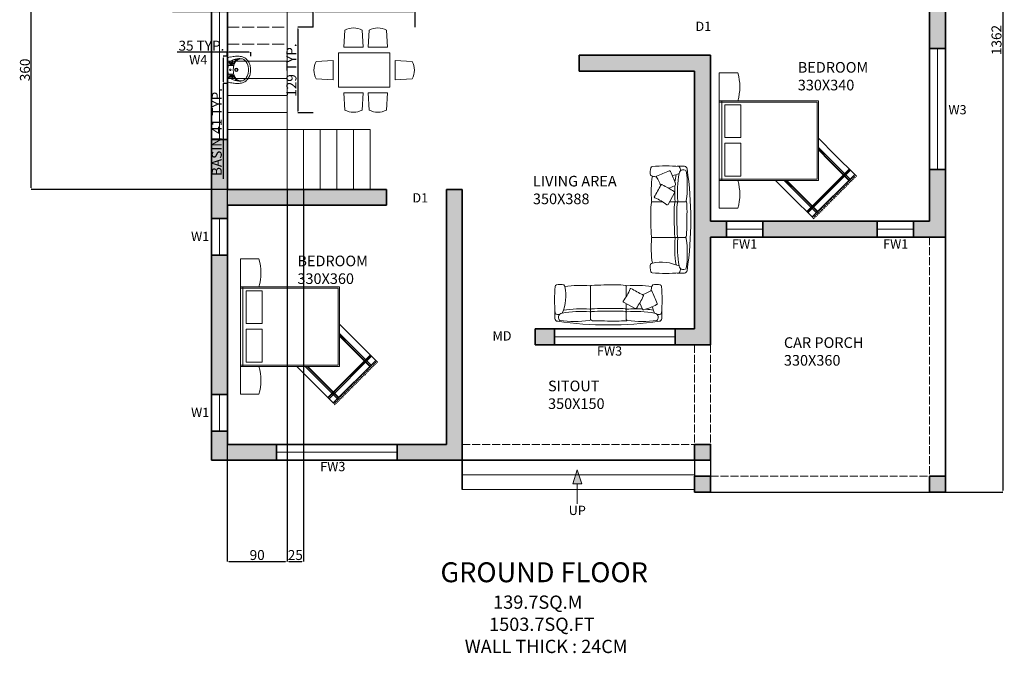
# Model space of a CAD drawing. Units: centimetres. Extents: x 2449 to 7478, y 778 to 2486.
# Tile 5 of 9: x 4189 to 5672, y 778 to 1732. Entities that reach past the tile are written whole.
import ezdxf

# ---------------------------------------------------------------- set-up
doc = ezdxf.new("R2010")
doc.units = ezdxf.units.CM
doc.linetypes.add('ACAD_ISO02W100', pattern=[15, 12, -3])
for name, color, linetype, lineweight in [('0.15', 34, 'Continuous', 15), ('A-ANNO-DIMS', 2, 'Continuous', 18), ('A-ANNO-SYMB', 8, 'Continuous', 18), ('A-ANNO-TEXT', 7, 'Continuous', 18), ('A-ANNO-TITL', 7, 'Continuous', 25), ('A-AREA-IDEN', 7, 'Continuous', 18), ('A-COLS', 7, 'Continuous', 35), ('A-COLS-PATT', 7, 'Continuous', 13), ('A-FLOR', 7, 'Continuous', 25), ('A-FLOR-FIXT', 8, 'Continuous', 18), ('A-FLOR-OVHD', 8, 'ACAD_ISO02W100', 18), ('A-FLOR-STRS', 7, 'Continuous', 18), ('A-FLOR-STRS-OVHD', 7, 'ACAD_ISO02W100', 13), ('A-WALL', 7, 'Continuous', 35), ('A-WALL-PATT', 7, 'Continuous', 13), ('B-FURNITURE', 22, 'Continuous', 18), ('Win', 1, 'Continuous', 18)]:
    doc.layers.add(name, color=color, linetype=linetype, lineweight=lineweight)
doc.styles.get("Standard").update_dxf_attribs({"font": 'arial.ttf'})
doc.dimstyles.new('ISO-25', dxfattribs={"dimtxt": 15, "dimasz": 2.5, "dimexe": 0, "dimexo": 0, "dimgap": 0, "dimtad": 1, "dimtxsty": 'Standard', "dimcen": 2.5, "dimadec": 0, "dimazin": 0, "dimtfac": 1, "dimtmove": 0, "dimatfit": 3, "dimfxl": 1, "dimarcsym": 0})

# ---------------------------------------------------------------- blocks, each defined once
blk = doc.blocks.new('ролар')
at = {"layer": 'B-FURNITURE'}
for p, q in [((182149, -12928), (182149, -13090)), ((182946, -12908), (182946, -13070)), ((183742, -12908), (183742, -13070)), ((184538, -12927), (184538, -13090)), ((182946, -13070), (182946, -13655)), ((183742, -13070), (183742, -13261)), ((183742, -13412), (183742, -13655))]:
    blk.add_line(p, q, dxfattribs=at)
blk.add_lwpolyline([(184124, -13426, 0.039108), (183972, -13160, 0.352413), (183942, -13151), (183685, -13293, 0.370087), (183675, -13320, -0.085318), (183831, -13592, 0.338149), (183848, -13604, -0.006963), (184118, -13456, 0.478074)], format="xyb", close=True, dxfattribs=at)
blk.add_lwpolyline([(184112, -13464, -0.054969), (184295, -13552, 0.338149), (184316, -13550, -0.006963), (184437, -13268, 0.478074), (184423, -13240, 0.039108), (184140, -13125, 0.352413), (184110, -13136), (184052, -13272)], format="xyb", dxfattribs=at)
for centre, radius, start, end in [((182209, -12928), 60, 90, 180), ((183344, -20690), 7904, 81.7476, 98.2524), ((182322, -12954), 95.7, 154.4132, 226.8965), ((182264, -12914), 28.1, 104.7154, 176.7534), ((182585, -15161), 2298, 81.7903, 98.2097), ((182918, -12915), 28.9, 15.2961, 99.1888), ((182999, -12942), 63.3, 99.7658, 147.0241), ((181568, 80195), 93085, 270.87421, 271.20678), ((183296, -20822), 7955, 86.6979, 88.3256), ((183770, -12915), 28.9, 80.8112, 164.7039), ((184102, -15161), 2298, 81.7903, 98.2097), ((184423, -12914), 28.1, 3.2466, 75.2846), ((184365, -12954), 95.7, 313.1035, 25.5868), ((184478, -12928), 60, 358.6006, 89.9879), ((186046, -13346), 3905, 175.5762, 184.4238), ((182224, -13128), 110, 72.3508, 130.321), ((182340, -12922), 131, 230.7956, 255.727), ((181452, -13440), 941, 347.608, 24.5904), ((182727, -10699), 2387, 259.8888, 274.8671), ((182725, -10712), 2434, 260.7796, 274.8194), ((182927, -13057), 20.3, 275.8765, 1.8), ((182927, -13117), 20.3, 275.8765, 1.8), ((182962, -13065), 17.3, 149.88, 272.0041), ((182962, -13125), 17.3, 149.88, 272.0041), ((183401, -6361), 6736, 266.2761, 271.089), ((183401, -6421), 6736, 266.2761, 271.089), ((183573, -12278), 819, 266.8813, 280.6931), ((183573, -12338), 819, 266.8813, 280.6931), ((183725, -13065), 17.3, 267.9959, 30.12), ((183725, -13125), 17.3, 267.9959, 30.12), ((183760, -13057), 20.3, 178.2, 264.1235), ((183760, -13117), 20.3, 178.2, 264.1235), ((183961, -10699), 2387, 265.1329, 280.1112), ((184001, -9721), 3425, 265.9379, 271.7664), ((184034, -11509), 1637, 275.2593, 281.2487), ((185235, -13440), 941, 155.4096, 164.8885), ((184348, -12922), 131, 284.273, 309.2044), ((184464, -13128), 110, 49.679, 107.6492), ((180641, -13346), 3905, 355.5762, 4.4238), ((182195, -13642), 42.7, 187.075, 250.1971), ((181903, -13435), 512, 330.8359, 336.0732), ((182722, -11168), 2503, 261.8987, 274.7524), ((182927, -13643), 20.3, 275.8765, 1.8), ((182962, -13651), 17.3, 149.88, 272.0041), ((183725, -13651), 17.3, 267.9959, 30.12), ((183760, -13643), 20.3, 178.2, 264.1235), ((183966, -11168), 2503, 265.2476, 278.1013), ((185235, -13440), 941, 186.9661, 192.392), ((184785, -13435), 512, 203.9268, 209.1641), ((184493, -13642), 42.7, 289.8029, 352.925), ((182270, -13358), 336, 254.5718, 283.8571), ((183401, -6946), 6736, 266.2761, 271.089), ((183573, -12863), 819, 266.8813, 280.6931), ((184418, -13358), 336, 256.1429, 285.4282)]:
    blk.add_arc(centre, radius, start, end, dxfattribs=at)
blk = doc.blocks.new('table-11')
at = {"color": 0, "linetype": 'ByBlock'}
for p, q in [((-1.122, 0.533), (-1.144, 0.134)), ((-0.716, 0.533), (-0.694, 0.134)), ((-0.554, 0.533), (-0.576, 0.134)), ((-0.148, 0.533), (-0.126, 0.134)), ((0, 0), (-1.2, 0)), ((-1.2, -0.8), (-1.2, 0)), ((-1.144, 0.134), (-0.694, 0.134)), ((-0.576, 0.134), (-0.126, 0.134)), ((0, -0.8), (0, 0)), ((-1.723, -0.197), (-1.324, -0.175)), ((-1.324, -0.625), (-1.324, -0.175)), ((0.523, -0.197), (0.124, -0.175)), ((0.124, -0.625), (0.124, -0.175)), ((-1.723, -0.603), (-1.324, -0.625)), ((0.523, -0.603), (0.124, -0.625)), ((0, -0.8), (-1.2, -0.8)), ((-1.144, -0.934), (-0.694, -0.934)), ((-1.122, -1.333), (-1.144, -0.934)), ((-0.716, -1.333), (-0.694, -0.934)), ((-0.576, -0.934), (-0.126, -0.934)), ((-0.554, -1.333), (-0.576, -0.934)), ((-0.148, -1.333), (-0.126, -0.934))]:
    blk.add_line(p, q, dxfattribs=at)
for centre, start, end in [((-0.919, 0.159), 61.4891, 118.5109), ((-0.351, 0.159), 61.4891, 118.5109), ((-1.349, -0.4), 151.4891, 208.5109), ((0.149, -0.4), 331.4891, 28.5109), ((-0.919, -0.959), 241.4891, 298.5109), ((-0.351, -0.959), 241.4891, 298.5109)]:
    blk.add_arc(centre, 0.425, start, end, dxfattribs=at)
blk = doc.blocks.new('A$C376C2187')
at = {"layer": 'B-FURNITURE'}
for p, q in [((-1.53, 1.82), (-1.53, 2.24)), ((-1.53, 2.24), (-0.9, 2.24)), ((-0.9, 0), (-0.9, 2.24)), ((-0.9, 2.24), (0.9, 2.24)), ((-0.9, 2.24), (-0.9, 1.82)), ((-0.87, 0.03), (-0.87, 2.24)), ((0.87, 2.24), (0.87, 0.03)), ((0.9, 2.24), (0.9, 0)), ((0.9, 1.82), (0.9, 2.24)), ((0.9, 2.24), (1.53, 2.24)), ((1.53, 2.24), (1.53, 1.82)), ((-0.9, 2.182), (0.9, 2.182)), ((-0.807, 2.112), (-0.057, 2.112)), ((-0.807, 1.749), (-0.807, 2.112)), ((-0.057, 2.112), (-0.057, 1.749)), ((0.069, 2.112), (0.807, 2.112)), ((0.069, 2.112), (0.069, 1.749)), ((0.807, 2.112), (0.807, 1.749)), ((-0.807, 1.749), (-0.057, 1.749)), ((0.069, 1.749), (0.807, 1.749)), ((0.9, 0), (-0.9, 0)), ((0.87, 0.03), (-0.87, 0.03))]:
    blk.add_line(p, q, dxfattribs=at)
for centre in [(-1.215, 2.926), (1.215, 2.926)]:
    blk.add_arc(centre, 1.15, 254.0965, 285.9035, dxfattribs=at)
blk = doc.blocks.new('lavamanos 2')
at = {"layer": '0.15'}
for p, q in [((0, 0.234), (0, -0.234)), ((-0.13, 0.11), (-0.131, 0.11)), ((-0.014, 0.087), (-0.13, 0.086)), ((-0.113, 0.112), (-0.107, 0.158)), ((-0.104, 0.111), (-0.098, 0.157)), ((-0.086, 0.109), (-0.081, 0.147)), ((-0.077, 0.107), (-0.072, 0.145)), ((-0.059, 0.105), (-0.055, 0.135)), ((-0.05, 0.104), (-0.046, 0.134)), ((-0.13, -0.11), (-0.131, -0.11)), ((-0.014, -0.087), (-0.13, -0.086)), ((-0.113, -0.112), (-0.107, -0.158)), ((-0.104, -0.111), (-0.098, -0.157)), ((-0.086, -0.109), (-0.081, -0.147)), ((-0.077, -0.107), (-0.072, -0.145)), ((-0.059, -0.105), (-0.055, -0.135)), ((-0.05, -0.104), (-0.046, -0.134))]:
    blk.add_line(p, q, dxfattribs=at)
for centre, radius in [((-0.178, 0), 0.035), ((-0.178, 0), 0.0235), ((-0.06, 0), 0.015)]:
    blk.add_circle(centre, radius, dxfattribs=at)
for centre, radius, start, end in [((-0.166, 0.001), 0.302, 136.5719, 154.3277), ((-0.242, 0.066), 0.202, 108.1945, 135.3686), ((-0.242, 0.065), 0.164, 121.9929, 150.5889), ((-0.266, 0.104), 0.119, 92.4774, 122.1411), ((-0.203, -0.086), 0.359, 91.203, 106.4255), ((-0.277, 0.068), 0.153, 57.2491, 95.54), ((-0.244, -0.013), 0.237, 77.2482, 96.4632), ((-0.221, -0.685), 0.959, 86.5514, 89.4131), ((-0.277, 0.068), 0.168, 56.8766, 64.9971), ((-0.222, 0.003), 0.218, 71.9849, 82.0124), ((-0.366, -0.002), 0.278, 40.3525, 49.2255), ((-0.212, -0.548), 0.82, 83.1224, 86.5796), ((-0.31, -0.315), 0.547, 69.5191, 73.4912), ((-0.299, -0.285), 0.516, 65.23, 69.5378), ((5.828, 30.215), 30.532, 258.7782, 258.876), ((-0.126, -0.066), 0.329, 69.0601, 78.8218), ((-0.02, 0.212), 0.0314, 54.7949, 69.0601), ((-0.005, 0.234), 0.005, 0, 54.7949), ((-0.209, 0.006), 0.256, 171.3102, 181.2627), ((-0.209, -0.006), 0.256, 178.7373, 188.6898), ((-0.056, -0.018), 0.411, 158.7011, 171.3102), ((0.466, -0.083), 0.895, 169.8632, 174.658), ((0.466, 0.083), 0.895, 185.342, 190.1368), ((-0.2, 0.026), 0.22, 147.1156, 167.4425), ((-0.366, -0.002), 0.263, 40.3525, 49.0046), ((-0.237, 0.11), 0.0921, 27.3186, 39.1156), ((-0.349, 0.036), 0.226, 22.3361, 30.8927), ((-0.237, 0.11), 0.107, 27.5743, 39.1156), ((-0.349, 0.036), 0.241, 22.1921, 30.7838), ((-1.266, -0.239), 1.182, 16.3631, 17.7767), ((-0.132, 0.117), 0.007, 197.4099, 270.4949), ((0.185, 0.165), 0.325, 192.5389, 196.7072), ((-0.13, 0.117), 0.007, 270.4949, 17.3953), ((-1.266, -0.239), 1.197, 17.3953, 17.8049), ((0.389, 0.121), 0.517, 185.5053, 189.8131), ((-0.718, -0.007), 0.599, 0.6765, 3.8216), ((-0.718, 0.007), 0.599, 356.1784, 359.3235), ((-0.108, 0.111), 0.0045, 172.614, 352.614), ((-0.102, 0.158), 0.0045, 352.614, 172.614), ((-0.081, 0.108), 0.0045, 172.614, 352.614), ((-0.278, -0.241), 0.466, 60.2413, 65.2382), ((-0.076, 0.146), 0.0045, 352.614, 172.614), ((-0.054, 0.104), 0.0045, 172.614, 352.614), ((-0.05, 0.135), 0.0045, 352.614, 172.614), ((-0.065, 0.118), 0.049, 1.5827, 68.6208), ((-2.148, 0.001), 2.135, 359.9754, 3.1901), ((-2.148, -0.001), 2.135, 356.8099, 0.0246), ((-0.056, 0.018), 0.411, 188.6898, 201.2989), ((-0.166, -0.001), 0.302, 205.6723, 223.4281), ((-0.2, -0.026), 0.22, 192.5575, 212.8844), ((-0.242, -0.065), 0.164, 209.4111, 238.0071), ((-0.277, -0.068), 0.153, 264.46, 302.7509), ((-0.366, 0.002), 0.263, 310.9954, 319.6475), ((-0.366, 0.002), 0.278, 310.7745, 319.6475), ((-0.237, -0.11), 0.0921, 320.8844, 332.6814), ((-0.349, -0.036), 0.226, 329.1073, 337.6639), ((-0.237, -0.11), 0.107, 320.8844, 332.4257), ((-0.349, -0.036), 0.241, 329.2162, 337.8079), ((-1.266, 0.239), 1.182, 342.2233, 343.6369), ((-0.132, -0.117), 0.007, 89.5051, 162.5901), ((0.185, -0.165), 0.325, 163.2928, 167.4611), ((-0.13, -0.117), 0.007, 342.6047, 89.5051), ((0.389, -0.121), 0.517, 170.1869, 174.4947), ((-1.266, 0.239), 1.197, 342.1951, 342.6047), ((-0.299, 0.286), 0.516, 290.4622, 294.77), ((-0.108, -0.111), 0.0045, 7.386, 187.386), ((-0.102, -0.158), 0.0045, 187.386, 7.386), ((-0.081, -0.108), 0.0045, 7.386, 187.386), ((-0.278, 0.241), 0.466, 294.7618, 299.7587), ((-0.076, -0.146), 0.0045, 187.386, 7.386), ((-0.054, -0.104), 0.0045, 7.386, 187.386), ((-0.05, -0.135), 0.0045, 187.386, 7.386), ((-0.065, -0.118), 0.049, 291.3792, 358.4173), ((-0.242, -0.066), 0.202, 224.6314, 251.8055), ((-0.266, -0.104), 0.119, 237.8589, 267.5226), ((-0.203, 0.086), 0.359, 253.5745, 268.797), ((-0.244, 0.013), 0.237, 263.5368, 282.7518), ((-0.221, 0.685), 0.959, 270.5869, 273.4486), ((-0.277, -0.068), 0.168, 295.0029, 303.1234), ((-0.222, -0.003), 0.218, 277.9876, 288.0151), ((-0.212, 0.548), 0.82, 273.4204, 276.8776), ((-0.31, 0.315), 0.547, 286.5088, 290.4809), ((5.828, -30.215), 30.532, 101.124, 101.2218), ((-0.126, 0.066), 0.329, 281.1782, 290.9399), ((-0.02, -0.212), 0.0314, 290.9399, 305.2051), ((-0.005, -0.234), 0.005, 305.2051, 0)]:
    blk.add_arc(centre, radius, start, end, dxfattribs=at)
blk = doc.blocks.new('RUG-FRINGED-B')
for p, q in [((90.4, 95.2), (64.4, 121.3)), ((64.4, 107.4), (83.5, 88.3)), ((64.4, 104.7), (82.1, 86.9)), ((64.4, 103.6), (81.6, 86.3)), ((90.4, 95.2), (119.1, 66.6)), ((110.7, 74.9), (46.8, 11)), ((111.3, 74.4), (47.4, 10.4)), ((110.2, 57.7), (81.6, 86.3)), ((110.8, 58.3), (82.1, 86.9)), ((112.1, 59.7), (83.5, 88.3)), ((112.7, 73), (48.7, 9)), ((119.1, 66.6), (55.1, 2.7)), ((112.3, 59.9), (115, 57.3)), ((114, 61.6), (116.6, 58.9)), ((115.7, 63.2), (118.3, 60.6)), ((117.4, 64.9), (120, 62.3)), ((119.1, 66.6), (121.7, 64)), ((0, 57.8), (26.5, 31.3)), ((32.9, 37.7), (12.8, 57.8)), ((34.2, 39), (15.5, 57.8)), ((34.8, 39.6), (16.7, 57.8)), ((97.2, 44.8), (99.8, 42.1)), ((98.9, 46.4), (101.5, 43.8)), ((100.6, 48.1), (103.2, 45.5)), ((102.3, 49.8), (104.9, 47.2)), ((103.9, 51.5), (106.6, 48.9)), ((105.6, 53.2), (108.2, 50.5)), ((107.3, 54.8), (109.9, 52.2)), ((109, 56.5), (111.6, 53.9)), ((110.7, 58.2), (113.3, 55.6)), ((55.1, 2.7), (26.5, 31.3)), ((32.9, 37.7), (61.5, 9)), ((34.2, 39), (62.9, 10.4)), ((34.8, 39.6), (63.4, 11)), ((83.8, 31.3), (86.4, 28.7)), ((85.5, 33), (88.1, 30.4)), ((87.1, 34.7), (89.8, 32.1)), ((88.8, 36.4), (91.4, 33.7)), ((90.5, 38), (93.1, 35.4)), ((92.2, 39.7), (94.8, 37.1)), ((93.9, 41.4), (96.5, 38.8)), ((95.5, 43.1), (98.2, 40.5)), ((68.7, 16.2), (71.3, 13.6)), ((70.3, 17.9), (73, 15.3)), ((72, 19.6), (74.6, 16.9)), ((73.7, 21.2), (76.3, 18.6)), ((75.4, 22.9), (78, 20.3)), ((77.1, 24.6), (79.7, 22)), ((78.7, 26.3), (81.4, 23.7)), ((80.4, 28), (83, 25.3)), ((82.1, 29.6), (84.7, 27)), ((55.2, 2.8), (57.8, 0.1)), ((56.9, 4.4), (59.5, 1.8)), ((58.6, 6.1), (61.2, 3.5)), ((60.3, 7.8), (62.9, 5.2)), ((61.9, 9.5), (64.6, 6.9)), ((63.6, 11.2), (66.2, 8.5)), ((65.3, 12.8), (67.9, 10.2)), ((67, 14.5), (69.6, 11.9))]:
    blk.add_line(p, q)
for centre in [(118.4, 60.6), (120.1, 62.2), (121.8, 63.9), (103.3, 45.4), (105, 47.1), (106.6, 48.8), (108.3, 50.5), (110, 52.2), (111.7, 53.8), (113.4, 55.5), (115, 57.2), (116.7, 58.9), (88.1, 30.3), (89.8, 32), (91.5, 33.7), (93.2, 35.4), (94.9, 37), (96.5, 38.7), (98.2, 40.4), (99.9, 42.1), (101.6, 43.8), (73, 15.2), (74.7, 16.9), (76.4, 18.6), (78.1, 20.2), (79.7, 21.9), (81.4, 23.6), (83.1, 25.3), (84.8, 27), (86.5, 28.6), (57.9, 0.1), (59.6, 1.8), (61.3, 3.4), (62.9, 5.1), (64.6, 6.8), (66.3, 8.5), (68, 10.2), (69.7, 11.8), (71.3, 13.5)]:
    blk.add_circle(centre, 0.0789)
blk = doc.blocks.new('ARROW-ENTRY-UP')
at = {"transparency": 33554687}
h = blk.add_hatch(color=256, dxfattribs=at)
h.dxf.hatch_style = 1
h.paths.add_polyline_path([(-6.8, 30.3), (6.8, 30.3), (0, 51.2)])
blk.add_line((0, 30.3), (0, 0))
blk.add_lwpolyline([(0, 51.2), (-6.8, 30.3), (6.8, 30.3)], close=True)
blk = doc.blocks.new('*D88')
at = {"layer": 'A-ANNO-DIMS', "color": 0, "lineweight": -2, "transparency": 16777216}
for p, q in [((4630.8, 1743.6), (4418.6, 1743.6)), ((4630.8, 1720.5), (4630.8, 1743.6)), ((4781.9, 1743.6), (4633.3, 1743.6)), ((4784.4, 1720.5), (4784.4, 1743.6))]:
    blk.add_line(p, q, dxfattribs=at)
at = {"layer": 'A-ANNO-DIMS', "color": 0, "transparency": 16777216}
for points in [[(4633.3, 1744), (4633.3, 1743.2), (4630.8, 1743.6)], [(4781.9, 1744), (4781.9, 1743.2), (4784.4, 1743.6)]]:
    blk.add_solid(points, dxfattribs=at)
at = {"layer": 'Defpoints', "color": 0, "transparency": 16777216}
for p in [(4630.8, 1743.6), (4630.8, 1720.5), (4784.4, 1720.5)]:
    blk.add_point(p, dxfattribs=at)
at = {"layer": 'A-ANNO-DIMS', "color": 0, "transparency": 16777216, "insert": (4523.4, 1751.3), "char_height": 15, "attachment_point": 5}
blk.add_mtext('DINING SET 154 TYP.', dxfattribs=at)
blk = doc.blocks.new('*D89')
at = {"layer": 'A-ANNO-DIMS', "color": 0, "lineweight": -2, "transparency": 16777216}
for p, q in [((4630.8, 1720.5), (4607.7, 1720.5)), ((4607.7, 1718), (4607.7, 1593.9)), ((4630.8, 1591.4), (4607.7, 1591.4))]:
    blk.add_line(p, q, dxfattribs=at)
at = {"layer": 'A-ANNO-DIMS', "color": 0, "transparency": 16777216}
for points in [[(4607.3, 1718), (4608.1, 1718), (4607.7, 1720.5)], [(4607.3, 1593.9), (4608.1, 1593.9), (4607.7, 1591.4)]]:
    blk.add_solid(points, dxfattribs=at)
at = {"layer": 'Defpoints', "color": 0, "transparency": 16777216}
for p in [(4630.8, 1720.5), (4607.7, 1591.4), (4630.8, 1591.4)]:
    blk.add_point(p, dxfattribs=at)
at = {"layer": 'A-ANNO-DIMS', "color": 0, "transparency": 16777216, "insert": (4600, 1656), "char_height": 15, "attachment_point": 5, "rotation": 90}
blk.add_mtext('129 TYP.', dxfattribs=at)
blk = doc.blocks.new('*D94')
at = {"layer": 'A-ANNO-DIMS', "color": 0, "lineweight": -2, "transparency": 16777216}
for p, q in [((4501.4, 1676.9), (4495.3, 1676.9)), ((4495.3, 1674.4), (4495.3, 1638.2)), ((4501.4, 1635.7), (4495.3, 1635.7)), ((4495.3, 1635.7), (4495.3, 1492.2))]:
    blk.add_line(p, q, dxfattribs=at)
at = {"layer": 'A-ANNO-DIMS', "color": 0, "transparency": 16777216}
for points in [[(4494.9, 1674.4), (4495.7, 1674.4), (4495.3, 1676.9)], [(4494.9, 1638.2), (4495.7, 1638.2), (4495.3, 1635.7)]]:
    blk.add_solid(points, dxfattribs=at)
at = {"layer": 'Defpoints', "color": 0, "transparency": 16777216}
for p in [(4501.4, 1676.9), (4495.3, 1635.7), (4501.4, 1635.7)]:
    blk.add_point(p, dxfattribs=at)
at = {"layer": 'A-ANNO-DIMS', "color": 0, "transparency": 16777216, "insert": (4487.5, 1562.7), "char_height": 15, "attachment_point": 5, "rotation": 89.9999}
blk.add_mtext('BASIN 41 TYP.', dxfattribs=at)
blk = doc.blocks.new('*D95')
at = {"layer": 'A-ANNO-DIMS', "color": 0, "lineweight": -2, "transparency": 16777216}
for p, q in [((4501.4, 1683.1), (4425.9, 1683.1)), ((4501.4, 1676.9), (4501.4, 1683.1)), ((4534.1, 1683.1), (4503.9, 1683.1)), ((4536.6, 1676.9), (4536.6, 1683.1))]:
    blk.add_line(p, q, dxfattribs=at)
at = {"layer": 'A-ANNO-DIMS', "color": 0, "transparency": 16777216}
for points in [[(4503.9, 1683.5), (4503.9, 1682.7), (4501.4, 1683.1)], [(4534.1, 1683.5), (4534.1, 1682.7), (4536.6, 1683.1)]]:
    blk.add_solid(points, dxfattribs=at)
at = {"layer": 'Defpoints', "color": 0, "transparency": 16777216}
for p in [(4501.4, 1683.1), (4501.4, 1676.9), (4536.6, 1676.9)]:
    blk.add_point(p, dxfattribs=at)
at = {"layer": 'A-ANNO-DIMS', "color": 0, "transparency": 16777216, "insert": (4462.4, 1690.8), "char_height": 15, "attachment_point": 5, "rotation": 359.9999}
blk.add_mtext('35 TYP.', dxfattribs=at)
blk = doc.blocks.new('*D101')
at = {"layer": 'A-ANNO-DIMS', "color": 0, "lineweight": -2, "transparency": 16777216}
for p, q in [((5583.4, 2382.3), (5669.9, 2382.3)), ((5669.9, 2379.8), (5669.9, 1022.8)), ((5583.4, 1020.3), (5669.9, 1020.3))]:
    blk.add_line(p, q, dxfattribs=at)
at = {"layer": 'A-ANNO-DIMS', "color": 0, "transparency": 16777216}
for points in [[(5669.5, 2379.8), (5670.4, 2379.8), (5669.9, 2382.3)], [(5669.5, 1022.8), (5670.4, 1022.8), (5669.9, 1020.3)]]:
    blk.add_solid(points, dxfattribs=at)
at = {"layer": 'Defpoints', "color": 0, "transparency": 16777216}
for p in [(5583.4, 2382.3), (5583.4, 1020.3), (5669.9, 1020.3)]:
    blk.add_point(p, dxfattribs=at)
at = {"layer": 'A-ANNO-DIMS', "color": 0, "transparency": 16777216, "insert": (5662.3, 1701.3), "char_height": 15, "attachment_point": 5, "rotation": 90}
blk.add_mtext('1362', dxfattribs=at)
blk = doc.blocks.new('*D102')
at = {"layer": 'A-ANNO-DIMS', "color": 0, "lineweight": -2, "transparency": 16777216}
for p, q in [((4501.4, 1476.3), (4501.4, 916)), ((4591.4, 1476.3), (4591.4, 916)), ((4503.9, 916), (4588.9, 916))]:
    blk.add_line(p, q, dxfattribs=at)
at = {"layer": 'A-ANNO-DIMS', "color": 0, "transparency": 16777216}
for points in [[(4503.9, 916.4), (4503.9, 915.6), (4501.4, 916)], [(4588.9, 916.4), (4588.9, 915.6), (4591.4, 916)]]:
    blk.add_solid(points, dxfattribs=at)
at = {"layer": 'Defpoints', "color": 0, "transparency": 16777216}
for p in [(4501.4, 1476.3), (4591.4, 1476.3), (4591.4, 916)]:
    blk.add_point(p, dxfattribs=at)
at = {"layer": 'A-ANNO-DIMS', "color": 0, "transparency": 16777216, "insert": (4546.4, 923.7), "char_height": 15, "attachment_point": 5}
blk.add_mtext('90', dxfattribs=at)
blk = doc.blocks.new('*D103')
at = {"layer": 'A-ANNO-DIMS', "color": 0, "lineweight": -2, "transparency": 16777216}
for p, q in [((4591.4, 1476.3), (4591.4, 916)), ((4616.4, 1476.3), (4616.4, 916)), ((4593.9, 916), (4613.9, 916))]:
    blk.add_line(p, q, dxfattribs=at)
at = {"layer": 'A-ANNO-DIMS', "color": 0, "transparency": 16777216}
for points in [[(4593.9, 916.4), (4593.9, 915.6), (4591.4, 916)], [(4613.9, 916.4), (4613.9, 915.6), (4616.4, 916)]]:
    blk.add_solid(points, dxfattribs=at)
at = {"layer": 'Defpoints', "color": 0, "transparency": 16777216}
for p in [(4591.4, 1476.3), (4616.4, 1476.3), (4616.4, 916)]:
    blk.add_point(p, dxfattribs=at)
at = {"layer": 'A-ANNO-DIMS', "color": 0, "transparency": 16777216, "insert": (4603.9, 923.7), "char_height": 15, "attachment_point": 5}
blk.add_mtext('25', dxfattribs=at)
blk = doc.blocks.new('*D104')
at = {"layer": 'A-ANNO-DIMS', "color": 0, "lineweight": -2, "transparency": 16777216}
for p, q in [((4501.4, 1836.3), (4206.1, 1836.3)), ((4206.1, 1478.8), (4206.1, 1833.8)), ((4501.4, 1476.3), (4206.1, 1476.3))]:
    blk.add_line(p, q, dxfattribs=at)
at = {"layer": 'A-ANNO-DIMS', "color": 0, "transparency": 16777216}
for points in [[(4205.7, 1833.8), (4206.5, 1833.8), (4206.1, 1836.3)], [(4205.7, 1478.8), (4206.5, 1478.8), (4206.1, 1476.3)]]:
    blk.add_solid(points, dxfattribs=at)
at = {"layer": 'Defpoints', "color": 0, "transparency": 16777216}
for p in [(4206.1, 1836.3), (4501.4, 1836.3), (4501.4, 1476.3)]:
    blk.add_point(p, dxfattribs=at)
at = {"layer": 'A-ANNO-DIMS', "color": 0, "transparency": 16777216, "insert": (4198.4, 1656.3), "char_height": 15, "attachment_point": 5, "rotation": 90}
blk.add_mtext('360', dxfattribs=at)

msp = doc.modelspace()

# ---------------------------------------------------------------- hatches: boundary and pattern name
at = {"layer": 'A-COLS-PATT'}
h = msp.add_hatch(color=256, dxfattribs=at)
h.dxf.hatch_style = 1
h.paths.add_polyline_path([(5229.448, 1092.34), (5205.448, 1092.34), (5205.448, 1068.34), (5229.448, 1068.34)])
h = msp.add_hatch(color=256, dxfattribs=at)
h.dxf.hatch_style = 1
h.paths.add_polyline_path([(5205.448, 1020.34), (5229.448, 1020.34), (5229.448, 1044.34), (5205.448, 1044.34)])
h = msp.add_hatch(color=256, dxfattribs=at)
h.dxf.hatch_style = 1
h.paths.add_polyline_path([(5559.448, 1020.34), (5583.448, 1020.34), (5583.448, 1044.34), (5559.448, 1044.34)])
at = {"layer": 'A-WALL-PATT'}
h = msp.add_hatch(color=256, dxfattribs=at)
h.dxf.hatch_style = 1
h.paths.add_polyline_path([(4831.448, 1092.34), (4757.448, 1092.34), (4757.448, 1068.34), (4855.448, 1068.34), (4855.448, 1476.34), (4831.448, 1476.34)])
h.paths.add_polyline_path([(4477.448, 1167.34), (4501.448, 1167.34), (4501.448, 1377.34), (4477.448, 1377.34)])
h.paths.add_polyline_path([(4575.448, 1068.34), (4575.448, 1092.34), (4501.448, 1092.34), (4501.448, 1112.34), (4477.448, 1112.34), (4477.448, 1068.34)])
h.paths.add_polyline_path([(4501.448, 1551.34), (4477.448, 1551.34), (4477.448, 1432.34), (4501.448, 1432.34), (4501.448, 1452.34), (4741.448, 1452.34), (4741.448, 1476.34), (4501.448, 1476.34)])
h.paths.add_polyline_path([(5205.448, 1654.34), (5205.448, 1266.34), (5176.448, 1266.34), (5176.448, 1242.34), (5229.448, 1242.34), (5229.448, 1404.34), (5253.448, 1404.34), (5253.448, 1428.34), (5229.448, 1428.34), (5229.448, 1678.34), (5031.448, 1678.34), (5031.448, 1654.34)])
h.paths.add_polyline_path([(4994.448, 1266.34), (4965.448, 1266.34), (4965.448, 1242.34), (4994.448, 1242.34)])
h.paths.add_polyline_path([(5583.448, 1506.339), (5559.448, 1506.339), (5559.448, 1428.34), (5535.448, 1428.34), (5535.448, 1404.34), (5583.448, 1404.34)])
h.paths.add_polyline_path([(5480.448, 1404.34), (5480.448, 1428.34), (5308.448, 1428.34), (5308.448, 1404.34)])
h.paths.add_polyline_path([(5559.448, 1688.339), (5583.448, 1688.339), (5583.448, 1826.34), (5559.448, 1826.34), (5559.448, 1792.34), (5418.448, 1792.34), (5418.448, 1768.34), (5559.448, 1768.34)])
h.paths.add_polyline_path([(5559.448, 1956.34), (5319.448, 1956.34), (5319.448, 1792.34), (5205.448, 1792.34), (5205.448, 1768.34), (5343.448, 1768.34), (5343.448, 1932.34), (5559.448, 1932.34), (5559.448, 1898.34), (5583.448, 1898.34), (5583.448, 2065.339), (5559.448, 2065.339)])
h.paths.add_polyline_path([(5559.448, 2358.34), (5559.448, 2247.339), (5583.448, 2247.339), (5583.448, 2382.34), (5535.448, 2382.34), (5535.448, 2358.34)])
h.paths.add_polyline_path([(5308.448, 2382.34), (5308.448, 2358.34), (5480.448, 2358.34), (5480.448, 2382.34)])
h.paths.add_polyline_path([(5229.448, 2358.34), (5253.448, 2358.34), (5253.448, 2382.34), (5205.448, 2382.34), (5205.448, 2214.34), (5166.448, 2214.34), (5166.448, 2190.34), (5205.448, 2190.34), (5205.448, 2065.34), (5229.448, 2065.34)])
h.paths.add_polyline_path([(5002.448, 2214.34), (5002.448, 2190.34), (5031.448, 2190.34), (5031.448, 1966.34), (5205.448, 1966.34), (5205.448, 1932.34), (5229.448, 1932.34), (5229.448, 1990.34), (5055.448, 1990.34), (5055.448, 2190.34), (5094.448, 2190.34), (5094.448, 2214.34)])
h.paths.add_polyline_path([(4901.448, 2190.34), (4930.448, 2190.34), (4930.448, 2214.34), (4803.448, 2214.34), (4803.448, 2190.34), (4877.448, 2190.34), (4877.448, 1836.34), (4901.448, 1836.34), (4901.448, 1966.34), (4956.448, 1966.34), (4956.448, 1990.34), (4901.448, 1990.34)])
h.paths.add_polyline_path([(4509.448, 2214.34), (4509.448, 2190.34), (4523.448, 2190.34), (4523.448, 1935.34), (4547.448, 1935.34), (4547.448, 2190.34), (4621.448, 2190.34), (4621.448, 2214.34)])
h.paths.add_polyline_path([(4349.448, 2152.839), (4373.448, 2152.839), (4373.448, 2190.34), (4387.448, 2190.34), (4387.448, 2214.34), (4349.448, 2214.34)])
h.paths.add_polyline_path([(4349.448, 1935.34), (4373.448, 1935.34), (4373.448, 1970.839), (4349.448, 1970.839)])
h.paths.add_polyline_path([(4477.448, 1836.34), (4477.448, 1791.34), (4501.448, 1791.34), (4501.448, 1836.34), (4787.448, 1836.34), (4787.448, 1860.34), (4349.448, 1860.34), (4349.448, 1836.34)])

# ---------------------------------------------------------------- linework, layer by layer
at = {"layer": 'A-COLS'}
for points in [[(5205.448, 1068.34), (5229.448, 1068.34), (5229.448, 1092.34), (5205.448, 1092.34)], [(5205.448, 1020.34), (5229.448, 1020.34), (5229.448, 1044.34), (5205.448, 1044.34)], [(5559.448, 1020.34), (5583.448, 1020.34), (5583.448, 1044.34), (5559.448, 1044.34)]]:
    msp.add_lwpolyline(points, close=True, dxfattribs=at)
at = {"layer": 'A-FLOR'}
for p, q in [((5205.448, 1092.34), (5205.448, 1020.34)), ((5229.448, 1092.34), (5229.448, 1044.34)), ((5205.448, 1044.34), (5229.448, 1044.34)), ((5205.448, 1020.34), (5583.448, 1020.34))]:
    msp.add_line(p, q, dxfattribs=at)
at = {"layer": 'A-FLOR-OVHD'}
for p, q in [((5559.448, 1404.34), (5559.448, 1044.34)), ((5205.448, 1242.34), (5205.448, 1092.34)), ((5229.448, 1242.34), (5229.448, 1092.34)), ((4855.448, 1092.34), (5229.448, 1092.34)), ((5229.448, 1044.34), (5559.448, 1044.34))]:
    msp.add_line(p, q, dxfattribs=at)
at = {"layer": 'A-FLOR-STRS'}
for p, q in [((4591.448, 1836.34), (4591.448, 1476.34)), ((4501.448, 1669.21), (4591.448, 1669.21)), ((4501.448, 1643.47), (4591.448, 1643.47)), ((4501.448, 1617.76), (4591.448, 1617.76)), ((4501.448, 1592.05), (4591.448, 1592.05)), ((4501.448, 1566.34), (4716.448, 1566.34)), ((4616.448, 1566.34), (4616.448, 1476.34)), ((4641.448, 1566.34), (4641.448, 1476.34)), ((4666.448, 1566.34), (4666.448, 1476.34)), ((4691.448, 1566.34), (4691.448, 1476.34)), ((4716.448, 1566.34), (4716.448, 1476.34)), ((4855.448, 1046.34), (5205.448, 1046.34)), ((4855.448, 1024.34), (5205.448, 1024.34))]:
    msp.add_line(p, q, dxfattribs=at)
at = {"layer": 'A-FLOR-STRS-OVHD', "ltscale": 1.5}
for p, q in [((4501.448, 1720.63), (4591.448, 1720.63)), ((4501.448, 1694.92), (4591.448, 1694.92))]:
    msp.add_line(p, q, dxfattribs=at)
at = {"layer": 'A-WALL'}
for p, q in [((5583.448, 2382.34), (5583.448, 1020.34)), ((4477.448, 1836.34), (4477.448, 1068.34)), ((4501.448, 1836.34), (4501.448, 1476.34)), ((5559.448, 1768.34), (5559.448, 1428.34)), ((5031.448, 1678.34), (5031.448, 1654.34)), ((5031.448, 1678.34), (5229.448, 1678.34)), ((5229.448, 1678.34), (5229.448, 1428.34)), ((5559.448, 1688.339), (5583.448, 1688.339)), ((5031.448, 1654.34), (5205.448, 1654.34)), ((5205.448, 1654.34), (5205.448, 1266.34)), ((4501.448, 1551.34), (4477.448, 1551.34)), ((5559.448, 1506.339), (5583.448, 1506.339)), ((4501.448, 1476.34), (4741.448, 1476.34)), ((4741.448, 1476.34), (4741.448, 1452.34)), ((4831.448, 1476.34), (4831.448, 1092.34)), ((4831.448, 1476.34), (4855.448, 1476.34)), ((4855.448, 1476.34), (4855.448, 1024.34)), ((4501.448, 1452.34), (4501.448, 1092.34)), ((4501.448, 1452.34), (4741.448, 1452.34)), ((4477.448, 1432.34), (4501.448, 1432.34)), ((5229.448, 1428.34), (5559.448, 1428.34)), ((5253.448, 1428.34), (5253.448, 1404.34)), ((5308.448, 1428.34), (5308.448, 1404.34)), ((5480.448, 1428.34), (5480.448, 1404.34)), ((5535.448, 1428.34), (5535.448, 1404.34)), ((5229.448, 1404.34), (5229.448, 1242.34)), ((5229.448, 1404.34), (5583.448, 1404.34)), ((4477.448, 1377.34), (4501.448, 1377.34)), ((4965.448, 1266.34), (4965.448, 1242.34)), ((4965.448, 1266.34), (5205.448, 1266.34)), ((4994.448, 1266.34), (4994.448, 1242.34)), ((5176.448, 1266.34), (5176.448, 1242.34)), ((4965.448, 1242.34), (5229.448, 1242.34)), ((4477.448, 1167.34), (4501.448, 1167.34)), ((4477.448, 1112.34), (4501.448, 1112.34)), ((4501.448, 1092.34), (4831.448, 1092.34)), ((4575.448, 1092.34), (4575.448, 1068.34)), ((4757.448, 1092.34), (4757.448, 1068.34)), ((4477.448, 1068.34), (5229.448, 1068.34))]:
    msp.add_line(p, q, dxfattribs=at)
at = {"layer": 'Win'}
for p, q in [((4489.448, 1791.34), (4489.448, 1551.34)), ((5571.448, 1688.339), (5571.448, 1506.339)), ((4489.448, 1432.34), (4489.448, 1377.34)), ((5253.448, 1416.34), (5308.448, 1416.34)), ((5480.448, 1416.34), (5535.448, 1416.34)), ((4994.448, 1254.34), (5176.448, 1254.34)), ((4489.448, 1112.34), (4489.448, 1167.34)), ((4575.448, 1080.34), (4757.448, 1080.34))]:
    msp.add_line(p, q, dxfattribs=at)

# ---------------------------------------------------------------- block references
at = {"layer": 'A-ANNO-SYMB'}
msp.add_blockref('ARROW-ENTRY-UP', (5028.72, 1002.514), dxfattribs=at)
at = {"layer": 'A-FLOR-FIXT', "xscale": 75.44223598555656, "yscale": 75.44223598555656, "zscale": 75.44223598555656, "rotation": 179.99990349049}
msp.add_blockref('lavamanos 2', (4501.448, 1656.34), dxfattribs=at)
at = {"layer": 'B-FURNITURE'}
for name, p, xscale, yscale, zscale, rotation in [('table-11', (4668.893, 1630.173), 64.48907140530227, 64.48907140530227, 64.48907140530227, 180), ('A$C376C2187', (5391.938, 1549.792), 66.63496932822166, 66.63496932822166, 66.63496932822166, 90), ('ролар', (6060.356, -10910.435), -0.0673113048210398, 0.0673113048210398, 0.0673113048210398, 270), ('A$C376C2187', (4670.396, 1269.652), 66.63496932822166, 66.63496932822166, 66.63496932822166, 90), ('ролар', (-7265.592, 411.556), -0.0673113048210398, 0.0673113048210398, 0.0673113048210398, 180)]:
    msp.add_blockref(name, p, dxfattribs=dict(at, xscale=xscale, yscale=yscale, zscale=zscale, rotation=rotation))
for p in [(5327.585, 1432.041), (4606.043, 1151.901)]:
    msp.add_blockref('RUG-FRINGED-B', p, dxfattribs=at)

# ---------------------------------------------------------------- texts
at = {"layer": 'A-ANNO-TEXT', "char_height": 14, "attachment_point": 1}
for s, insert in [('{\\fTimes New Roman|b0|i0|c0|p18;\\PD1}', (5206.838, 1752.244)), ('{\\fTimes New Roman|b0|i0|c0|p18;\\PW4}', (4443.972, 1701.978)), ('{\\fTimes New Roman|b0|i0|c0|p18;\\PW3}', (5587.953, 1626.636)), ('{\\fTimes New Roman|b0|i0|c0|p18;\\PD1}', (4780.33, 1493.941)), ('{\\fTimes New Roman|b0|i0|c0|p18;\\PW1}', (4446.836, 1435.743)), ('{\\fTimes New Roman|b0|i0|c0|p18;\\PFW1}', (5261.889, 1424.402)), ('{\\fTimes New Roman|b0|i0|c0|p18;\\PFW1}', (5489.56, 1424.402)), ('{\\fTimes New Roman|b0|i0|c0|p18;\\PMD}', (4900.997, 1286.053)), ('{\\fTimes New Roman|b0|i0|c0|p18;\\PFW3}', (5058.462, 1263.247)), ('{\\fTimes New Roman|b0|i0|c0|p18;\\PW1}', (4446.836, 1170.743)), ('{\\fTimes New Roman|b0|i0|c0|p18;\\PFW3}', (4641.385, 1089.247)), ('{\\fTimes New Roman|b0|i0|c0|p18;\\PUP}', (5015.813, 1023.213))]:
    msp.add_mtext_dynamic_manual_height_columns(s, width=211.90348, gutter_width=12.5, heights=[0], dxfattribs=dict(at, insert=insert))
at = {"layer": 'A-ANNO-TITL', "insert": (4822.561, 914.668), "char_height": 30, "attachment_point": 1}
msp.add_mtext_dynamic_manual_height_columns('{\\fTimes New Roman|b0|i0|c0|p18;GROUND FLOOR\\P\\H0.66667x;             139.7SQ.M\\P            1503.7SQ.FT\\P      WALL THICK : 24CM}', width=483.87687, gutter_width=12.5, heights=[0], dxfattribs=at)
at = {"layer": 'A-AREA-IDEN', "char_height": 16, "attachment_point": 1}
for s, insert in [('{\\fTimes New Roman|b0|i0|c0|p18;\\PBEDROOM           330X340}', (5360.946, 1694.796)), ('{\\fTimes New Roman|b0|i0|c0|p18;\\PLIVING AREA             350X388}', (4961.928, 1523.391)), ('{\\fTimes New Roman|b0|i0|c0|p18;\\PBEDROOM           330X360}', (4607.061, 1403.202)), ('{\\fTimes New Roman|b0|i0|c0|p18;\\PCAR PORCH  330X360}', (5340.073, 1280.209)), ('{\\fTimes New Roman|b0|i0|c0|p18;\\PSITOUT           350X150}', (4984.663, 1214.933))]:
    msp.add_mtext_dynamic_manual_height_columns(s, width=211.90348, gutter_width=12.5, heights=[0], dxfattribs=dict(at, insert=insert))

# ---------------------------------------------------------------- dimensions: what is measured, and where the dimension line sits
at = {"layer": 'A-ANNO-DIMS'}
for base, p1, p2, picture, middle in [((5669.948, 1020.34), (5583.448, 2382.34), (5583.448, 1020.34), '*D101', (5662.284, 1701.34)), ((4206.091, 1836.34), (4501.448, 1476.34), (4501.448, 1836.34), '*D104', (4198.428, 1656.34))]:
    dim = msp.add_linear_dim(base=base, p1=p1, p2=p2, angle=90, dimstyle='ISO-25', override={"dimdec": 0, "dimlfac": 1, "dimrnd": 0, "dimzin": 0, "dimdsep": 46, "dimlunit": 2}, dxfattribs=at)
    dim.commit()
    dim.dimension.update_dxf_attribs({"geometry": picture, "text_midpoint": middle})
for base, p1, p2, angle, text, picture, middle in [((4630.751, 1743.594), (4784.422, 1720.543), (4630.751, 1720.543), 180, 'DINING SET <> TYP.', '*D88', (4523.42, 1751.35)), ((4501.448, 1683.114), (4536.553, 1676.935), (4501.448, 1676.935), 179.999903, '<> TYP.', '*D95', (4462.445, 1690.778)), ((4607.701, 1591.395), (4630.751, 1720.543), (4630.751, 1591.395), 270, '<> TYP.', '*D89', (4600.042, 1655.969)), ((4495.269, 1635.744), (4501.448, 1676.935), (4501.448, 1635.744), 269.999903, 'BASIN <> TYP.', '*D94', (4487.513, 1562.715))]:
    dim = msp.add_linear_dim(base=base, p1=p1, p2=p2, angle=angle, text=text, dimstyle='ISO-25', override={"dimdec": 0, "dimlfac": 1, "dimrnd": 0, "dimzin": 0, "dimdsep": 46, "dimlunit": 2}, dxfattribs=at)
    dim.commit()
    dim.dimension.update_dxf_attribs({"geometry": picture, "text_midpoint": middle})
for base, p1, p2, picture, middle in [((4591.448, 916.014), (4501.448, 1476.34), (4591.448, 1476.34), '*D102', (4546.448, 923.672)), ((4616.448, 916.014), (4591.448, 1476.34), (4616.448, 1476.34), '*D103', (4603.948, 923.672))]:
    dim = msp.add_linear_dim(base=base, p1=p1, p2=p2, dimstyle='ISO-25', override={"dimdec": 0, "dimlfac": 1, "dimrnd": 0, "dimzin": 0, "dimdsep": 46, "dimlunit": 2}, dxfattribs=at)
    dim.commit()
    dim.dimension.update_dxf_attribs({"geometry": picture, "text_midpoint": middle})

doc.saveas('drawing.dxf')
